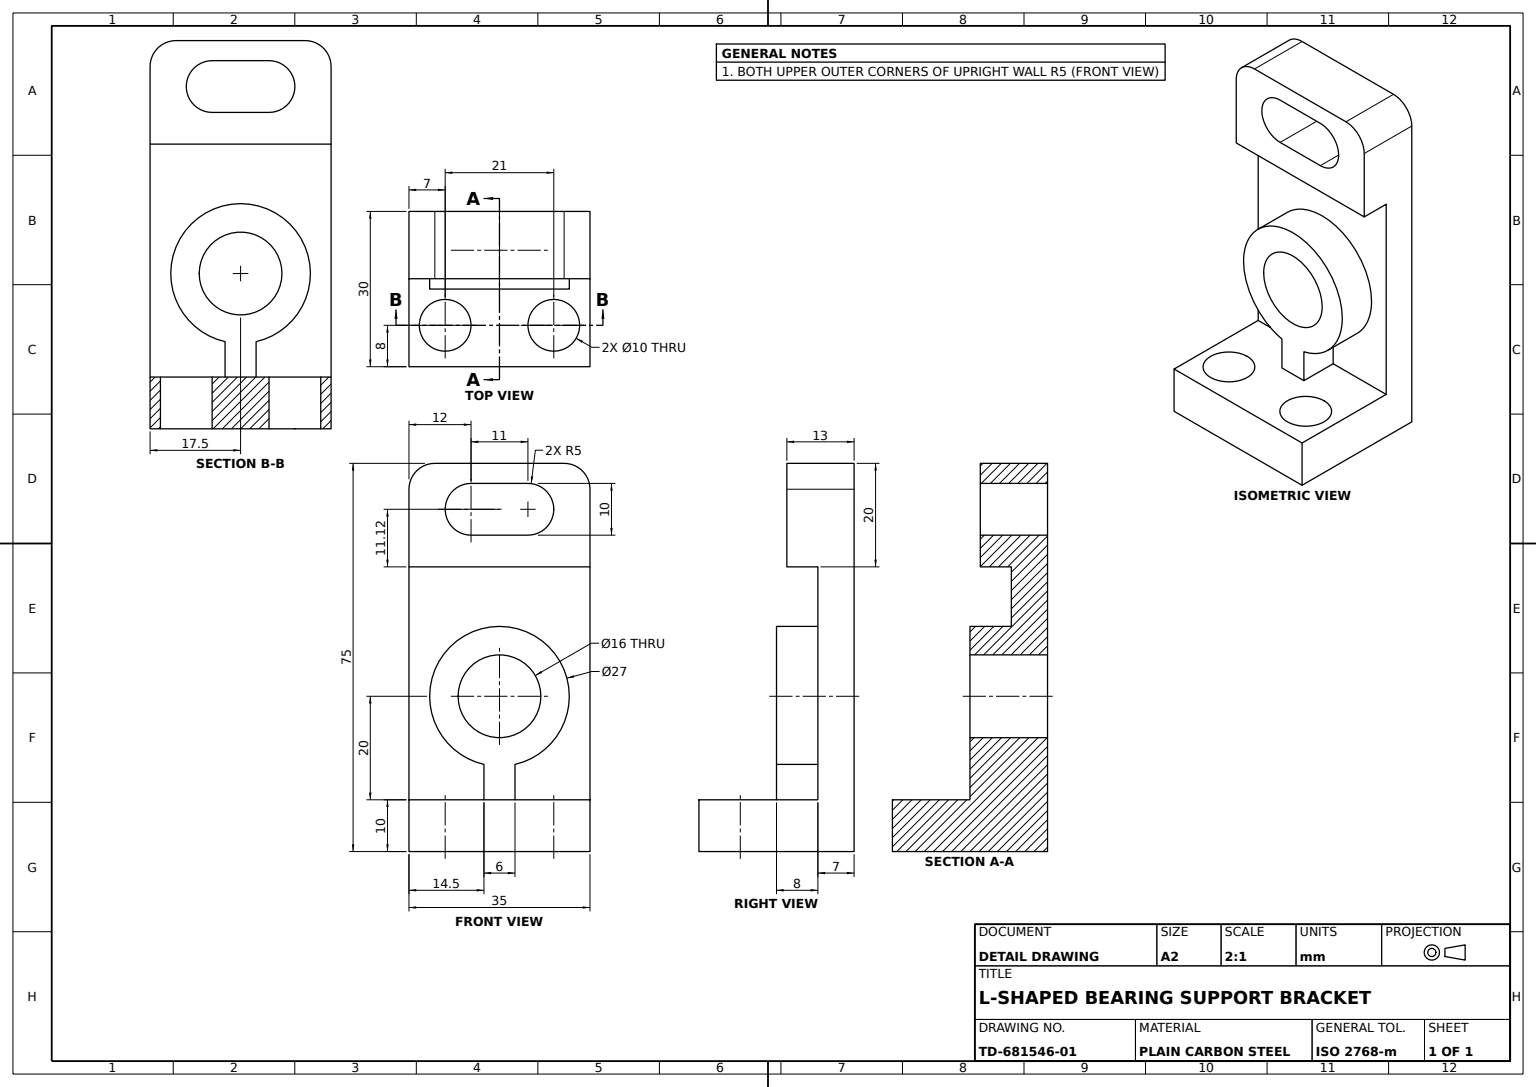
from build123d import *

# Parameters (mm, degrees)
BASE_PLATE_SKETCH_W      = 35
BASE_PLATE_SKETCH_H      = 30
BASE_PLATE_DEPTH         = 10
UPRIGHT_WALL_SKETCH_W    = 35
UPRIGHT_WALL_SKETCH_H    = 7
UPRIGHT_WALL_DEPTH       = 65
TOP_PAD_SKETCH_W         = 35
TOP_PAD_SKETCH_H         = 20
TOP_PAD_DEPTH            = 6
WALL_MOUNTING_SLOT_DEPTH = 13
BEARING_BOSS_SKETCH_R    = 8
BEARING_BOSS_DEPTH       = 8
BASE_HOLE_A_SKETCH_R     = 5
BASE_HOLE_A_DEPTH        = 10
BASE_HOLE_B_SKETCH_R     = 5
BASE_HOLE_B_DEPTH        = 10
BEARING_START            = -10
BEARING_BORE_SKETCH_R    = 8
BEARING_BORE_DEPTH       = 10
WALL_TOP_FILLET_R5_A_R   = 5
WALL_TOP_FILLET_R5_B_R   = 5


with BuildPart() as part:
    # Base Plate Sketch → Base Plate (new body)
    with BuildSketch(Plane(origin=(0, 0, 0), x_dir=(1, 0, 0), z_dir=(0, 1, 0))):
        Rectangle(BASE_PLATE_SKETCH_W, BASE_PLATE_SKETCH_H)
    extrude(amount=BASE_PLATE_DEPTH)

    # Upright Wall Sketch → Upright Wall (add)
    with BuildSketch(Plane(origin=(0, 10, 0), x_dir=(1, 0, 0), z_dir=(0, 1, 0))):
        with Locations((0, 11.5)):
            Rectangle(UPRIGHT_WALL_SKETCH_W, UPRIGHT_WALL_SKETCH_H)
    extrude(amount=UPRIGHT_WALL_DEPTH)

    # Top Pad Sketch → Top Pad (add)
    with BuildSketch(Plane.XY.offset(-8)):
        with Locations((0, 65)):
            Rectangle(TOP_PAD_SKETCH_W, TOP_PAD_SKETCH_H)
    extrude(amount=TOP_PAD_DEPTH)

    # Wall Mounting Slot Sketch → Wall Mounting Slot (cut)
    with BuildSketch(Plane.XY.offset(-2)):
        with BuildLine():
            Line((-5.5, 71.124987094), (5.5, 71.124987094))
            ThreePointArc((5.5, 71.124987094), (10.5, 66.124987094), (5.5, 61.124987094))
            Line((5.5, 61.124987094), (-5.5, 61.124987094))
            ThreePointArc((-5.5, 61.124987094), (-10.5, 66.124987094), (-5.5, 71.124987094))
        make_face()
    extrude(amount=-WALL_MOUNTING_SLOT_DEPTH, mode=Mode.SUBTRACT)

    # Bearing Boss Sketch → Bearing Boss (add)
    with BuildSketch(Plane.XY.offset(-8)):
        with BuildLine():
            Line((-3, 16.837553419), (-3, 10))
            Line((-3, 10), (3, 10))
            Line((3, 10), (3, 16.837553419))
            ThreePointArc((3, 16.837553419), (0, 43.5), (-3, 16.837553419))
        make_face()
        with Locations((0, 30)):
            Circle(BEARING_BOSS_SKETCH_R, mode=Mode.SUBTRACT)
    extrude(amount=BEARING_BOSS_DEPTH)

    # Base Hole A Sketch → Base Hole A (cut)
    with BuildSketch(Plane(origin=(0, 10, 0), x_dir=(1, 0, 0), z_dir=(0, 1, 0))):
        with Locations(Location((-10.5, -7, 0), (0, 0, 270))):
            Circle(BASE_HOLE_A_SKETCH_R)
    extrude(amount=-BASE_HOLE_A_DEPTH, mode=Mode.SUBTRACT)

    # Base Hole B Sketch → Base Hole B (cut)
    with BuildSketch(Plane(origin=(0, 10, 0), x_dir=(1, 0, 0), z_dir=(0, 1, 0))):
        with Locations(Location((10.5, -7, 0), (0, 0, 270))):
            Circle(BASE_HOLE_B_SKETCH_R)
    extrude(amount=-BASE_HOLE_B_DEPTH, mode=Mode.SUBTRACT)

    # Bearing Bore Sketch → Bearing Bore (cut)
    with BuildSketch(Plane.XY.offset(-8).offset(BEARING_START)):
        with Locations((0, 30)):
            Circle(BEARING_BORE_SKETCH_R)
    extrude(amount=BEARING_BORE_DEPTH, mode=Mode.SUBTRACT)

    # Wall Top Fillet R5 A
    wall_top_fillet_r5_a_edges = [part.edges().sort_by_distance(p)[0] for p in [
        (-17.5, 75, -8.5),
    ]]
    fillet(wall_top_fillet_r5_a_edges, radius=WALL_TOP_FILLET_R5_A_R)

    # Wall Top Fillet R5 B
    wall_top_fillet_r5_b_edges = [part.edges().sort_by_distance(p)[0] for p in [
        (17.5, 75, -8.5),
    ]]
    fillet(wall_top_fillet_r5_b_edges, radius=WALL_TOP_FILLET_R5_B_R)


solid = part.part
